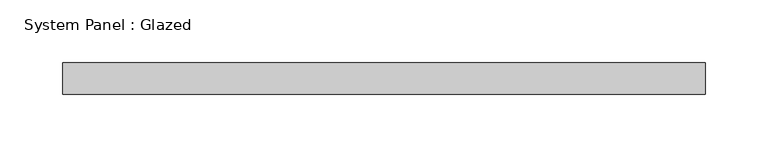
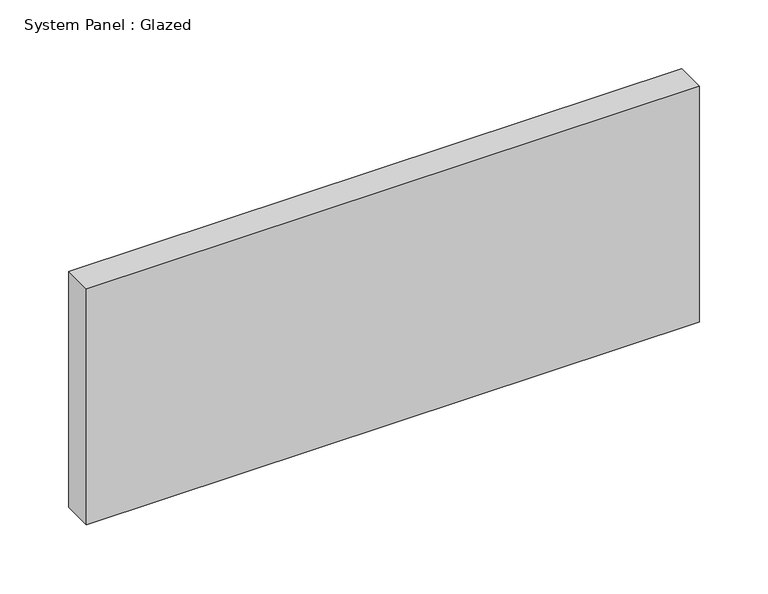
"""IFC4 building model written with IfcOpenShell, lengths in millimetres: plate geometry, System Panel : Glazed."""

from ifc_helpers import new_model, si_unit, origin, origin_with_axes, place, context, project, spatial, polyline, outline, extrude, source, transform, mapped, element, save


def system_panel_glazed_63160b6e(model_context):
    return source(origin(), model_context, "Body", "SweptSolid", [
        extrude(outline(polyline([(257.175, 19.05), (-257.175, 19.05), (-257.175, 44.45), (257.175, 44.45), (257.175, 19.05)])), origin_with_axes(), (0.0, 0.0, 1.0), 209.55),
    ])


if __name__ == "__main__":
    model = new_model("IFC4")
    model_context = context("Model", 3, world=origin())
    ifc_project = project(units=[si_unit("LENGTHUNIT", "METRE", prefix="MILLI")], contexts=[model_context])
    site = spatial("IfcSite", under=ifc_project)
    building = spatial("IfcBuilding", under=site)
    placement = place(None, origin())
    system_panel_glazed_shape = system_panel_glazed_63160b6e(model_context)
    element("IfcPlate", 1, ObjectType="System Panel : Glazed", at=placement, inside=building, context=model_context, shape_type="MappedRepresentation", body=[
        mapped(system_panel_glazed_shape, transform((0.0, 0.0, 0.0), x_axis=(1.0, 0.0, 0.0), y_axis=(0.0, 1.0, 0.0), z_axis=(0.0, 0.0, 1.0))),
    ])
    save(model, "model.ifc")

# Revit data of these elements
# Type "System Panel : Glazed"
#   Construction Type Id = "GSP4R"
#   Analytic Construction = "1/8 in Pilkington single glazing"
#   Visual Light Transmittance = 0.9
#   Solar Heat Gain Coefficient = 0.86
#   Heat Transfer Coefficient (U) = 1.18115 BTU/(h·ft²·°F)
#   Define Thermal Properties by = 1
# Element 1 (IfcPlate, "System Panel : Glazed")
#   Materials on its faces: "Glass"
# Materials
#   "Glass": class "Glass", colour RGB 0 128 192, transparency 0.75, Description = "Soda Lime Glass", Cost = 0
